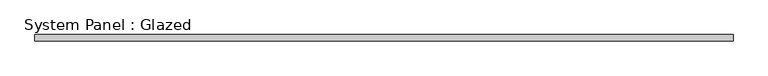
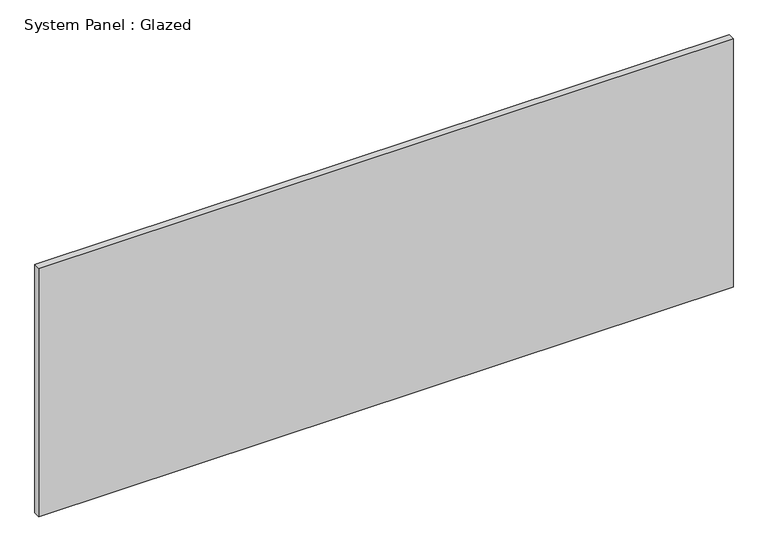
"""IFC4 building model written with IfcOpenShell, lengths in millimetres: plate geometry, System Panel : Glazed."""

from ifc_helpers import new_model, si_unit, origin, origin_with_axes, place, context, project, spatial, polyline, outline, extrude, source, transform, mapped, element, save


def system_panel_glazed_a729a16e(model_context):
    return source(origin(), model_context, "Body", "SweptSolid", [
        extrude(outline(polyline([(1337.475, 24.5), (-1337.475, 24.5), (-1337.475, 49.5), (1337.475, 49.5), (1337.475, 24.5)])), origin_with_axes(), (0.0, 0.0, 1.0), 1012.218874),
    ])


if __name__ == "__main__":
    model = new_model("IFC4")
    model_context = context("Model", 3, world=origin())
    ifc_project = project(units=[si_unit("LENGTHUNIT", "METRE", prefix="MILLI")], contexts=[model_context])
    site = spatial("IfcSite", under=ifc_project)
    building = spatial("IfcBuilding", under=site)
    placement = place(None, origin())
    system_panel_glazed_shape = system_panel_glazed_a729a16e(model_context)
    element("IfcPlate", 1, ObjectType="System Panel : Glazed", at=placement, inside=building, context=model_context, shape_type="MappedRepresentation", body=[
        mapped(system_panel_glazed_shape, transform((0.0, 0.0, 0.0), x_axis=(1.0, 0.0, 0.0), y_axis=(0.0, 1.0, 0.0), z_axis=(0.0, 0.0, 1.0))),
    ])
    save(model, "model.ifc")

# Revit data of these elements
# Type "System Panel : Glazed"
#   Keynote = "H11"
#   Construction Type Id = "GSP4R"
#   Analytic Construction = "1/8 in Pilkington single glazing"
#   Visual Light Transmittance = 0.9
#   Solar Heat Gain Coefficient = 0.86
#   Heat Transfer Coefficient (U) = 6.7069 W/(m²·K)
#   Define Thermal Properties by = 1
# Element 1 (IfcPlate, "System Panel : Glazed")
#   Materials on its faces: "Glass"
# Materials
#   "Glass": class "Glass", colour RGB 0 128 192, transparency 0.9, Description = "Soda Lime Glass", Cost = 0
